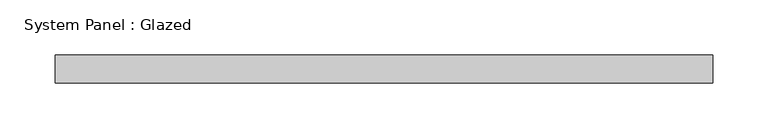
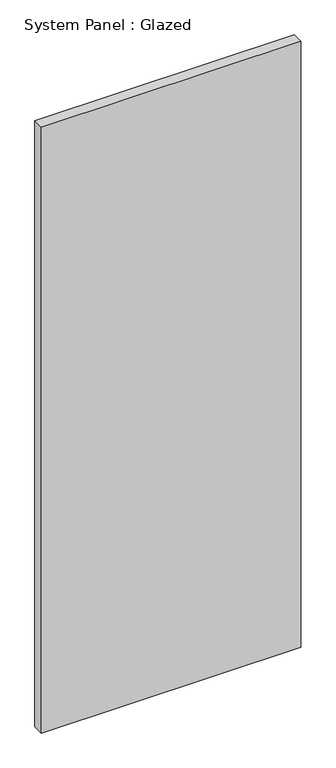
"""IFC4 building model written with IfcOpenShell, lengths in millimetres: plate geometry, System Panel : Glazed."""

from ifc_helpers import new_model, si_unit, origin, origin_with_axes, place, context, project, spatial, polyline, outline, extrude, source, transform, mapped, element, save


def system_panel_glazed_761c0abc(model_context):
    return source(origin(), model_context, "Body", "SweptSolid", [
        extrude(outline(polyline([(298.45, 19.05), (-298.45, 19.05), (-298.45, 44.45), (298.45, 44.45), (298.45, 19.05)])), origin_with_axes(), (0.0, 0.0, 1.0), 1474.4580508),
    ])


if __name__ == "__main__":
    model = new_model("IFC4")
    model_context = context("Model", 3, world=origin())
    ifc_project = project(units=[si_unit("LENGTHUNIT", "METRE", prefix="MILLI")], contexts=[model_context])
    site = spatial("IfcSite", under=ifc_project)
    building = spatial("IfcBuilding", under=site)
    placement = place(None, origin())
    system_panel_glazed_shape = system_panel_glazed_761c0abc(model_context)
    element("IfcPlate", 1, ObjectType="System Panel : Glazed", at=placement, inside=building, context=model_context, shape_type="MappedRepresentation", body=[
        mapped(system_panel_glazed_shape, transform((0.0, 0.0, 0.0), x_axis=(1.0, 0.0, 0.0), y_axis=(0.0, 1.0, 0.0), z_axis=(0.0, 0.0, 1.0))),
    ])
    save(model, "model.ifc")

# Revit data of these elements
# Type "System Panel : Glazed"
#   Construction Type Id = "GSP4R"
#   Analytic Construction = "1/8 in Pilkington single glazing"
#   Visual Light Transmittance = 0.9
#   Solar Heat Gain Coefficient = 0.86
#   Heat Transfer Coefficient (U) = 1.18115 BTU/(h·ft²·°F)
#   Define Thermal Properties by = 1
# Element 1 (IfcPlate, "System Panel : Glazed")
#   Materials on its faces: "Glass"
# Materials
#   "Glass": class "Glass", colour RGB 0 128 192, transparency 0.75, Description = "Soda Lime Glass", Cost = 0
